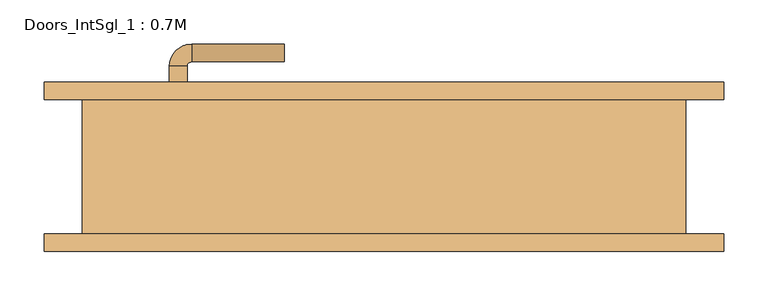
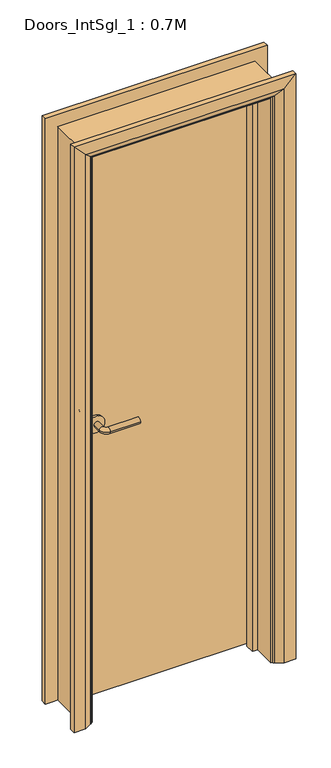
"""IFC4 building model written with IfcOpenShell, lengths in millimetres: door geometry, Doors_IntSgl_1 : 0.7M."""

from ifc_helpers import new_model, si_unit, point, frame, frame_2d, origin, place, context, project, spatial, polyline, circle_curve, ellipse_curve, trimmed, segment, composite_curve, outline, extrude, faceted_brep, source, transform, mapped, element, save
from ifc_brep_helpers import plane_surface, cylinder_surface, revolved_surface, advanced_brep


def doors_intsgl_1_0_7m_00cad461(model_context):
    return source(origin(), model_context, "Body", "SolidModel", [
        advanced_brep(
        [(-243.0, 30.2, 1000.0), (-223.0, 30.2, 1000.0), (-223.0, 0.2, 1000.0), (-243.0, 0.2, 1000.0), (-218.0, -4.8, 1000.0), (-218.0, -24.8, 1000.0), (-113.0, -24.8, 1000.0), (-113.0, -4.8, 1000.0)],
        [
            (0, 1, circle_curve(frame((-233.0, 30.2, 1000.0), z_axis=(0.0, 1.0, 0.0), x_axis=(1.0, 0.0, 0.0)), 10.0)),
            (1, 0, circle_curve(frame((-233.0, 30.2, 1000.0), z_axis=(0.0, 1.0, 0.0), x_axis=(1.0, 0.0, 0.0)), 10.0)),
            (1, 2),
            (2, 3, circle_curve(frame((-233.0, 0.2, 1000.0), z_axis=(0.0, 1.0, 0.0), x_axis=(1.0, 0.0, 0.0)), 10.0)),
            (3, 0),
            (3, 2, circle_curve(frame((-233.0, 0.2, 1000.0), z_axis=(0.0, 1.0, 0.0), x_axis=(1.0, 0.0, 0.0)), 10.0)),
            (4, 5, circle_curve(frame((-218.0, -14.8, 1000.0), z_axis=(-1.0, 0.0, 0.0), x_axis=(0.0, 1.0, 0.0)), 10.0)),
            (5, 3, circle_curve(frame((-218.0, 0.2, 1000.0), z_axis=(0.0, 0.0, -1.0), x_axis=(-1.0, 0.0, 0.0)), 25.0)),
            (2, 4, circle_curve(frame((-218.0, 0.2, 1000.0), z_axis=(0.0, 0.0, 1.0), x_axis=(-1.0, 0.0, 0.0)), 5.0)),
            (5, 4, circle_curve(frame((-218.0, -14.8, 1000.0), z_axis=(-1.0, 0.0, 0.0), x_axis=(0.0, 1.0, 0.0)), 10.0)),
            (6, 7, circle_curve(frame((-113.0, -14.8, 1000.0), z_axis=(1.0, 0.0, 0.0), x_axis=(0.0, 1.0, 0.0)), 10.0)),
            (7, 6, circle_curve(frame((-113.0, -14.8, 1000.0), z_axis=(1.0, 0.0, 0.0), x_axis=(0.0, 1.0, 0.0)), 10.0)),
            (4, 7),
            (6, 5),
        ],
        [
            plane_surface(frame((-233.0, 30.2, 1000.0), z_axis=(0.0, 1.0, 0.0), x_axis=(0.0, 0.0, 1.0))),
            cylinder_surface(frame((-233.0, 30.2, 1000.0), z_axis=(0.0, 1.0, 0.0), x_axis=(1.0, 0.0, 0.0)), 10.0),
            revolved_surface(trimmed(ellipse_curve(frame((-233.0, 0.2, 1000.0), z_axis=(0.0, -1.0, 0.0), x_axis=(1.0, 0.0, 0.0)), 10.0, 10.0), [point((-243.0, 0.2, 1000.0))], [point((-223.0, 0.2, 1000.0))], True, "CARTESIAN"), (-218.0, 0.2, 1000.0), (0.0, 0.0, -1.0)),
            revolved_surface(trimmed(ellipse_curve(frame((-233.0, 0.2, 1000.0), z_axis=(0.0, -1.0, 0.0), x_axis=(1.0, 0.0, 0.0)), 10.0, 10.0), [point((-223.0, 0.2, 1000.0))], [point((-243.0, 0.2, 1000.0))], True, "CARTESIAN"), (-218.0, 0.2, 1000.0), (0.0, 0.0, -1.0)),
            plane_surface(frame((-113.0, -14.8, 1000.0), z_axis=(1.0, 0.0, 0.0), x_axis=(0.0, 0.0, 1.0))),
            cylinder_surface(frame((-218.0, -14.8, 1000.0), z_axis=(-1.0, 0.0, 0.0), x_axis=(0.0, 1.0, 0.0)), 10.0),
        ],
        [
            (0, [[1, 2]]),
            (1, [[3, 4, 5, -2]]),
            (1, [[-5, 6, -3, -1]]),
            (2, [[7, 8, -4, 9]]),
            (3, [[10, -9, -6, -8]]),
            (4, [[11, 12]]),
            (5, [[13, -11, 14, -7]]),
            (5, [[-14, -12, -13, -10]]),
        ],
    ),
        extrude(outline(composite_curve([segment(trimmed(circle_curve(frame_2d((1000.0, -235.5)), 30.0), [point((1000.0, -265.5))], [point((1000.0, -205.5))], False, "CARTESIAN"), True, "CONTINUOUS"), segment(trimmed(circle_curve(frame_2d((1000.0, -235.5)), 30.0), [point((1000.0, -205.5))], [point((1000.0, -265.5))], False, "CARTESIAN"), True, "CONTINUOUS")], self_intersect=False)), frame((0.0, 30.2, 0.0), z_axis=(0.0, 1.0, 0.0), x_axis=(0.0, 0.0, 1.0)), (0.0, 0.0, 1.0), 8.0),
        advanced_brep(
        [(-243.0, 84.2, 1000.0), (-223.0, 84.2, 1000.0), (-243.0, 114.2, 1000.0), (-223.0, 114.2, 1000.0), (-218.0, 119.2, 1000.0), (-218.0, 139.2, 1000.0), (-113.0, 139.2, 1000.0), (-113.0, 119.2, 1000.0)],
        [
            (0, 1, circle_curve(frame((-233.0, 84.2, 1000.0), z_axis=(0.0, -1.0, 0.0), x_axis=(1.0, 0.0, 0.0)), 10.0)),
            (1, 0, circle_curve(frame((-233.0, 84.2, 1000.0), z_axis=(0.0, -1.0, 0.0), x_axis=(1.0, 0.0, 0.0)), 10.0)),
            (0, 2),
            (2, 3, circle_curve(frame((-233.0, 114.2, 1000.0), z_axis=(0.0, -1.0, 0.0), x_axis=(1.0, 0.0, 0.0)), 10.0)),
            (3, 1),
            (3, 2, circle_curve(frame((-233.0, 114.2, 1000.0), z_axis=(0.0, -1.0, 0.0), x_axis=(1.0, 0.0, 0.0)), 10.0)),
            (4, 3, circle_curve(frame((-218.0, 114.2, 1000.0), z_axis=(0.0, 0.0, 1.0), x_axis=(-1.0, 0.0, 0.0)), 5.0)),
            (2, 5, circle_curve(frame((-218.0, 114.2, 1000.0), z_axis=(0.0, 0.0, -1.0), x_axis=(-1.0, 0.0, 0.0)), 25.0)),
            (5, 4, circle_curve(frame((-218.0, 129.2, 1000.0), z_axis=(-1.0, 0.0, 0.0), x_axis=(0.0, -1.0, 0.0)), 10.0)),
            (4, 5, circle_curve(frame((-218.0, 129.2, 1000.0), z_axis=(-1.0, 0.0, 0.0), x_axis=(0.0, -1.0, 0.0)), 10.0)),
            (6, 7, circle_curve(frame((-113.0, 129.2, 1000.0), z_axis=(1.0, 0.0, 0.0), x_axis=(0.0, -1.0, 0.0)), 10.0)),
            (7, 6, circle_curve(frame((-113.0, 129.2, 1000.0), z_axis=(1.0, 0.0, 0.0), x_axis=(0.0, -1.0, 0.0)), 10.0)),
            (5, 6),
            (7, 4),
        ],
        [
            plane_surface(frame((-233.0, 84.2, 1000.0), z_axis=(0.0, -1.0, 0.0), x_axis=(0.0, 0.0, 1.0))),
            cylinder_surface(frame((-233.0, 84.2, 1000.0), z_axis=(0.0, -1.0, 0.0), x_axis=(1.0, 0.0, 0.0)), 10.0),
            revolved_surface(trimmed(ellipse_curve(frame((-233.0, 114.2, 1000.0), z_axis=(0.0, -1.0, 0.0), x_axis=(1.0, 0.0, 0.0)), 10.0, 10.0), [point((-243.0, 114.2, 1000.0))], [point((-223.0, 114.2, 1000.0))], True, "CARTESIAN"), (-218.0, 114.2, 1000.0), (0.0, 0.0, -1.0)),
            revolved_surface(trimmed(ellipse_curve(frame((-233.0, 114.2, 1000.0), z_axis=(0.0, -1.0, 0.0), x_axis=(1.0, 0.0, 0.0)), 10.0, 10.0), [point((-223.0, 114.2, 1000.0))], [point((-243.0, 114.2, 1000.0))], True, "CARTESIAN"), (-218.0, 114.2, 1000.0), (0.0, 0.0, -1.0)),
            plane_surface(frame((-113.0, 129.2, 1000.0), z_axis=(1.0, 0.0, 0.0), x_axis=(0.0, 0.0, 1.0))),
            cylinder_surface(frame((-218.0, 129.2, 1000.0), z_axis=(-1.0, 0.0, 0.0), x_axis=(0.0, -1.0, 0.0)), 10.0),
        ],
        [
            (0, [[1, 2]]),
            (1, [[-1, 3, 4, 5]]),
            (1, [[-2, -5, 6, -3]]),
            (2, [[7, -4, 8, 9]]),
            (3, [[-8, -6, -7, 10]]),
            (4, [[11, 12]]),
            (5, [[-9, 13, -12, 14]]),
            (5, [[-10, -14, -11, -13]]),
        ],
    ),
        extrude(outline(composite_curve([segment(trimmed(circle_curve(frame_2d((1000.0, -235.5)), 30.0), [point((1000.0, -265.5))], [point((1000.0, -205.5))], False, "CARTESIAN"), True, "CONTINUOUS"), segment(trimmed(circle_curve(frame_2d((1000.0, -235.5)), 30.0), [point((1000.0, -205.5))], [point((1000.0, -265.5))], False, "CARTESIAN"), True, "CONTINUOUS")], self_intersect=False)), frame((0.0, 76.2, 0.0), z_axis=(0.0, 1.0, 0.0), x_axis=(0.0, 0.0, 1.0)), (0.0, 0.0, 1.0), 8.0),
        extrude(outline(polyline([(308.0, 38.2), (-308.0, 38.2), (-308.0, 76.2), (308.0, 76.2), (308.0, 38.2)])), frame((0.0, 0.0, 8.0), z_axis=(0.0, 0.0, 1.0), x_axis=(1.0, 0.0, 0.0)), (0.0, 0.0, 1.0), 2060.0),
        faceted_brep([(-310.0, 76.2, 0.0), (-310.0, -76.2, 0.0), (-342.0, -76.2, 0.0), (-342.0, 76.2, 0.0), (-310.0, 76.2, 2070.0), (-310.0, -76.2, 2070.0), (-342.0, -76.2, 2102.0), (-342.0, 76.2, 2102.0), (310.0, 76.2, 0.0), (342.0, 76.2, 0.0), (342.0, -76.2, 0.0), (310.0, -76.2, 0.0), (310.0, 76.2, 2070.0), (342.0, 76.2, 2102.0), (342.0, -76.2, 2102.0), (310.0, -76.2, 2070.0)], [[[0, 1, 2, 3]], [[1, 0, 4, 5]], [[2, 1, 5, 6]], [[3, 2, 6, 7]], [[0, 3, 7, 4]], [[8, 9, 10, 11]], [[12, 13, 9, 8]], [[13, 14, 10, 9]], [[14, 15, 11, 10]], [[15, 12, 8, 11]], [[5, 4, 12, 15]], [[6, 5, 15, 14]], [[7, 6, 14, 13]], [[4, 7, 13, 12]]]),
        advanced_brep(
        [(-385.0, -96.2, 0.0), (-385.0, -76.2, 0.0), (-315.0, -76.2, 0.0), (-319.0, -82.2, 0.0), (-345.0, -96.2, 0.0), (-385.0, -96.2, 2145.0), (-385.0, -76.2, 2145.0), (-315.0, -76.2, 2075.0), (-319.0, -82.2, 2079.0), (-345.0, -96.2, 2105.0), (385.0, -96.2, 0.0), (345.0, -96.2, 0.0), (319.0, -82.2, 0.0), (315.0, -76.2, 0.0), (385.0, -76.2, 0.0), (385.0, -96.2, 2145.0), (345.0, -96.2, 2105.0), (319.0, -82.2, 2079.0), (315.0, -76.2, 2075.0), (385.0, -76.2, 2145.0)],
        [
            (0, 1),
            (1, 2),
            (2, 3, circle_curve(frame((-323.0, -75.2, 0.0), z_axis=(0.0, 0.0, -1.0), x_axis=(-1.0, 0.0, 0.0)), 8.0622577)),
            (3, 4),
            (4, 0),
            (0, 5),
            (5, 6),
            (6, 1),
            (6, 7),
            (7, 2),
            (7, 8, ellipse_curve(frame((-323.0, -75.2, 2083.0), z_axis=(-0.7071067811865475, 0.0, -0.7071067811865475), x_axis=(0.7071067811865474, 0.0, -0.7071067811865476)), 11.4017543, 8.0622577)),
            (8, 3),
            (8, 9),
            (9, 4),
            (9, 5),
            (10, 11),
            (11, 12),
            (12, 13, circle_curve(frame((323.0, -75.2, 0.0), z_axis=(0.0, 0.0, -1.0), x_axis=(1.0, 0.0, 0.0)), 8.0622577)),
            (13, 14),
            (14, 10),
            (15, 16),
            (16, 11),
            (10, 15),
            (16, 17),
            (17, 12),
            (17, 18, ellipse_curve(frame((323.0, -75.2, 2083.0), z_axis=(0.7071067811865475, 0.0, -0.7071067811865475), x_axis=(0.7071067811865474, 0.0, 0.7071067811865476)), 11.4017543, 8.0622577)),
            (18, 13),
            (18, 19),
            (19, 14),
            (19, 15),
            (5, 15),
            (19, 6),
            (18, 7),
            (17, 8),
            (16, 9),
        ],
        [
            plane_surface(frame((-315.0, -149.0010989, 0.0), z_axis=(0.0, 0.0, -1.0), x_axis=(1.0, 0.0, 0.0))),
            plane_surface(frame((-385.0, -96.2, 0.0), z_axis=(-1.0, 0.0, 0.0), x_axis=(0.0, 0.0, 1.0))),
            plane_surface(frame((-385.0, -76.2, 0.0), z_axis=(0.0, 1.0, 0.0), x_axis=(0.0, 0.0, 1.0))),
            cylinder_surface(frame((-323.0, -75.2, 0.0), z_axis=(0.0, 0.0, -1.0), x_axis=(-1.0, 0.0, 0.0)), 8.0622577),
            plane_surface(frame((-319.0, -82.2, 0.0), z_axis=(0.4740998230350183, -0.8804710999221749, 0.0), x_axis=(0.0, 0.0, 1.0))),
            plane_surface(frame((-345.0, -96.2, 0.0), z_axis=(0.0, -1.0, 0.0), x_axis=(0.0, 0.0, 1.0))),
            plane_surface(frame((315.0, -149.0010989, 0.0), z_axis=(0.0, 0.0, -1.0), x_axis=(-1.0, 0.0, 0.0))),
            plane_surface(frame((345.0, -96.2, 2105.0), z_axis=(0.0, -1.0, 0.0), x_axis=(0.0, 0.0, -1.0))),
            plane_surface(frame((319.0, -82.2, 2079.0), z_axis=(-0.4740998230350183, -0.8804710999221749, 0.0), x_axis=(0.0, 0.0, -1.0))),
            cylinder_surface(frame((323.0, -75.2, 2075.0), z_axis=(0.0, 0.0, 1.0), x_axis=(1.0, 0.0, 0.0)), 8.0622577),
            plane_surface(frame((385.0, -76.2, 2145.0), z_axis=(0.0, 1.0, 0.0), x_axis=(0.0, 0.0, -1.0))),
            plane_surface(frame((385.0, -96.2, 2145.0), z_axis=(1.0, 0.0, 0.0), x_axis=(0.0, 0.0, -1.0))),
            plane_surface(frame((-385.0, -96.2, 2145.0), z_axis=(0.0, 0.0, 1.0), x_axis=(1.0, 0.0, 0.0))),
            plane_surface(frame((-385.0, -76.2, 2145.0), z_axis=(0.0, 1.0, 0.0), x_axis=(1.0, 0.0, 0.0))),
            cylinder_surface(frame((-315.0, -75.2, 2083.0), z_axis=(-1.0, 0.0, 0.0), x_axis=(0.0, 0.0, 1.0)), 8.0622577),
            plane_surface(frame((-319.0, -82.2, 2079.0), z_axis=(0.0, -0.8804710999221749, -0.4740998230350183), x_axis=(1.0, 0.0, 0.0))),
            plane_surface(frame((-345.0, -96.2, 2105.0), z_axis=(0.0, -1.0, 0.0), x_axis=(1.0, 0.0, 0.0))),
        ],
        [
            (0, [[1, 2, 3, 4, 5]]),
            (1, [[-1, 6, 7, 8]]),
            (2, [[-2, -8, 9, 10]]),
            (3, [[-3, -10, 11, 12]]),
            (4, [[-4, -12, 13, 14]]),
            (5, [[-5, -14, 15, -6]]),
            (6, [[16, 17, 18, 19, 20]]),
            (7, [[21, 22, -16, 23]]),
            (8, [[24, 25, -17, -22]]),
            (9, [[26, 27, -18, -25]]),
            (10, [[28, 29, -19, -27]]),
            (11, [[30, -23, -20, -29]]),
            (12, [[-7, 31, -30, 32]]),
            (13, [[-9, -32, -28, 33]]),
            (14, [[-11, -33, -26, 34]]),
            (15, [[-13, -34, -24, 35]]),
            (16, [[-15, -35, -21, -31]]),
        ],
    ),
        extrude(outline(polyline([(0.0, -310.0), (0.0, -291.0), (2051.0, -291.0), (2051.0, 291.0), (0.0, 291.0), (0.0, 310.0), (2070.0, 310.0), (2070.0, -310.0), (0.0, -310.0)])), frame((0.0, 4.2, 0.0), z_axis=(0.0, 1.0, 0.0), x_axis=(0.0, 0.0, 1.0)), (0.0, 0.0, 1.0), 32.0),
        advanced_brep(
        [(385.0, 96.2, 0.0), (385.0, 76.2, 0.0), (315.0, 76.2, 0.0), (319.0, 82.2, 0.0), (345.0, 96.2, 0.0), (385.0, 96.2, 2145.0), (385.0, 76.2, 2145.0), (-385.0, 76.2, 2145.0), (-385.0, 76.2, 0.0), (-315.0, 76.2, 0.0), (-315.0, 76.2, 2075.0), (315.0, 76.2, 2075.0), (319.0, 82.2, 2079.0), (345.0, 96.2, 2105.0), (-345.0, 96.2, 2105.0), (-345.0, 96.2, 0.0), (-385.0, 96.2, 0.0), (-385.0, 96.2, 2145.0), (-319.0, 82.2, 0.0), (-319.0, 82.2, 2079.0)],
        [
            (0, 1),
            (1, 2),
            (2, 3, circle_curve(frame((323.0, 75.2, 0.0), z_axis=(0.0, 0.0, -1.0), x_axis=(1.0, 0.0, 0.0)), 8.0622577)),
            (3, 4),
            (4, 0),
            (0, 5),
            (5, 6),
            (6, 1),
            (6, 7),
            (7, 8),
            (8, 9),
            (9, 10),
            (10, 11),
            (11, 2),
            (11, 12, ellipse_curve(frame((323.0, 75.2, 2083.0), z_axis=(0.7071067811865475, 0.0, -0.7071067811865475), x_axis=(-0.7071067811865474, 0.0, -0.7071067811865476)), 11.4017543, 8.0622577)),
            (12, 3),
            (12, 13),
            (13, 4),
            (13, 14),
            (14, 15),
            (15, 16),
            (16, 17),
            (17, 5),
            (7, 17),
            (16, 8),
            (15, 18),
            (18, 9, circle_curve(frame((-323.0, 75.2, 0.0), z_axis=(0.0, 0.0, -1.0), x_axis=(-1.0, 0.0, 0.0)), 8.0622577)),
            (19, 10, ellipse_curve(frame((-323.0, 75.2, 2083.0), z_axis=(-0.7071067811865475, 0.0, -0.7071067811865475), x_axis=(-0.7071067811865474, 0.0, 0.7071067811865476)), 11.4017543, 8.0622577)),
            (18, 19),
            (14, 19),
            (19, 12),
        ],
        [
            plane_surface(frame((315.0, 76.2, 0.0), z_axis=(0.0, 0.0, -1.0), x_axis=(0.0, -1.0, 0.0))),
            plane_surface(frame((385.0, 96.2, 0.0), z_axis=(1.0, 0.0, 0.0), x_axis=(0.0, 0.0, 1.0))),
            plane_surface(frame((385.0, 76.2, 0.0), z_axis=(0.0, -1.0, 0.0), x_axis=(0.0, 0.0, 1.0))),
            cylinder_surface(frame((323.0, 75.2, 0.0), z_axis=(0.0, 0.0, -1.0), x_axis=(1.0, 0.0, 0.0)), 8.0622577),
            plane_surface(frame((319.0, 82.2, 0.0), z_axis=(-0.4740998230350126, 0.880471099922178, 0.0), x_axis=(0.0, 0.0, 1.0))),
            plane_surface(frame((345.0, 96.2, 0.0), z_axis=(0.0, 1.0, 0.0), x_axis=(0.0, 0.0, 1.0))),
            plane_surface(frame((-385.0, 96.2, 2145.0), z_axis=(-1.0, 0.0, 0.0), x_axis=(0.0, 0.0, -1.0))),
            plane_surface(frame((-315.0, 76.2, 0.0), z_axis=(0.0, 0.0, -1.0), x_axis=(0.0, -1.0, 0.0))),
            cylinder_surface(frame((-323.0, 75.2, 2075.0), z_axis=(0.0, 0.0, 1.0), x_axis=(-1.0, 0.0, 0.0)), 8.0622577),
            plane_surface(frame((-319.0, 82.2, 2079.0), z_axis=(0.47409982303501824, 0.8804710999221749, 0.0), x_axis=(0.0, 0.0, -1.0))),
            plane_surface(frame((385.0, 96.2, 2145.0), z_axis=(0.0, 0.0, 1.0), x_axis=(-1.0, 0.0, 0.0))),
            cylinder_surface(frame((315.0, 75.2, 2083.0), z_axis=(1.0, 0.0, 0.0), x_axis=(0.0, 0.0, 1.0)), 8.0622577),
            plane_surface(frame((319.0, 82.2, 2079.0), z_axis=(0.0, 0.8804710999221764, -0.4740998230350154), x_axis=(-1.0, 0.0, 0.0))),
        ],
        [
            (0, [[1, 2, 3, 4, 5]]),
            (1, [[-1, 6, 7, 8]]),
            (2, [[-2, -8, 9, 10, 11, 12, 13, 14]]),
            (3, [[-3, -14, 15, 16]]),
            (4, [[-4, -16, 17, 18]]),
            (5, [[-5, -18, 19, 20, 21, 22, 23, -6]]),
            (6, [[24, -22, 25, -10]]),
            (7, [[-21, 26, 27, -11, -25]]),
            (8, [[28, -12, -27, 29]]),
            (9, [[30, -29, -26, -20]]),
            (10, [[-7, -23, -24, -9]]),
            (11, [[-15, -13, -28, 31]]),
            (12, [[-17, -31, -30, -19]]),
        ],
    ),
    ])


if __name__ == "__main__":
    model = new_model("IFC4")
    model_context = context("Model", 3, world=origin())
    ifc_project = project(units=[si_unit("LENGTHUNIT", "METRE", prefix="MILLI")], contexts=[model_context])
    site = spatial("IfcSite", under=ifc_project)
    building = spatial("IfcBuilding", under=site)
    placement = place(None, origin())
    doors_intsgl_1_0_7m_shape = doors_intsgl_1_0_7m_00cad461(model_context)
    element("IfcDoor", 1, ObjectType="Doors_IntSgl_1 : 0.7M", at=placement, inside=building, context=model_context, shape_type="MappedRepresentation", body=[
        mapped(doors_intsgl_1_0_7m_shape, transform((0.0, 0.0, 0.0), x_axis=(1.0, 0.0, 0.0), y_axis=(0.0, 1.0, 0.0), z_axis=(0.0, 0.0, 1.0))),
    ])
    save(model, "model.ifc")

# Revit data of these elements
# Type "Doors_IntSgl_1 : 0.7M"
#   Type Mark = "58"
#   Type Comments = "Internal Single"
#   Operation = "SingleSwingRight"
#   Construction Type Id = "MDOOR"
#   Manufacturer = "Revit"
#   Keynote = "L20"
#   Description = "Internal Single Door"
#   Analytic Construction = "Metal"
#   UnderCut = 0.008 m
#   Tolerance = 0.002 m
#   Thickness = 0.038 m
#   Structural Tolerance = 0.008 m
#   StopDepth = 0.032 m
#   Stop Thickness = 0.019 m
#   Rough Width = 0.7 m
#   Rough Height = 2.11 m
#   Height to Top Lock Rail = 1.0 m
#   Heat Transfer Coefficient (U) = 3.7021 W/(m²·K)
#   Handle Z Distance = 1.0 m
#   Handle X Distance = 0.075 m
#   Frame Thickness = 0.032 m
#   Door Panel Width = 0.616 m
#   Door Panel Thickness = 0.038 m
#   Door Panel Offset = 0.0 m
#   Height = 2.11 m
#   Width = 0.7 m
#   Door Panel Height = 2.06 m
#   Architrave Setback = 0.005 m
#   Vis - Ironmongery = yes
#   Define Thermal Properties by = 1
#   Material Ironmongery = Door - Handle
#   Material Frame = Door - Frame/Mullion
#   Material Door = Door - Panel
#   Material Architrave = Door - Architrave
#   Visual Light Transmittance = 0
#   Solar Heat Gain Coefficient = 0
#   Function = (empty or 0)
#   Wall Closure = (empty or 0)
# Element 1 (IfcDoor, "Doors_IntSgl_1 : 0.7M")
#   Materials on its faces: "Door - Architrave", "Door - Handle", "Door - Frame/Mullion", "Door - Panel"
# Materials
#   "Door - Handle": colour RGB 0 0 0, transparency 0, Keynote = "P21", Cost = 0
#   "Door - Frame/Mullion": class "Wood", colour RGB 212 179 113, transparency 0, Keynote = "L20", Cost = 0
#   "Door - Panel": class "Wood", colour RGB 210 159 95, transparency 0, Keynote = "L20", Cost = 0
#   "Door - Architrave": class "Wood", colour RGB 154 90 5, transparency 0, Keynote = "P20", Cost = 0
